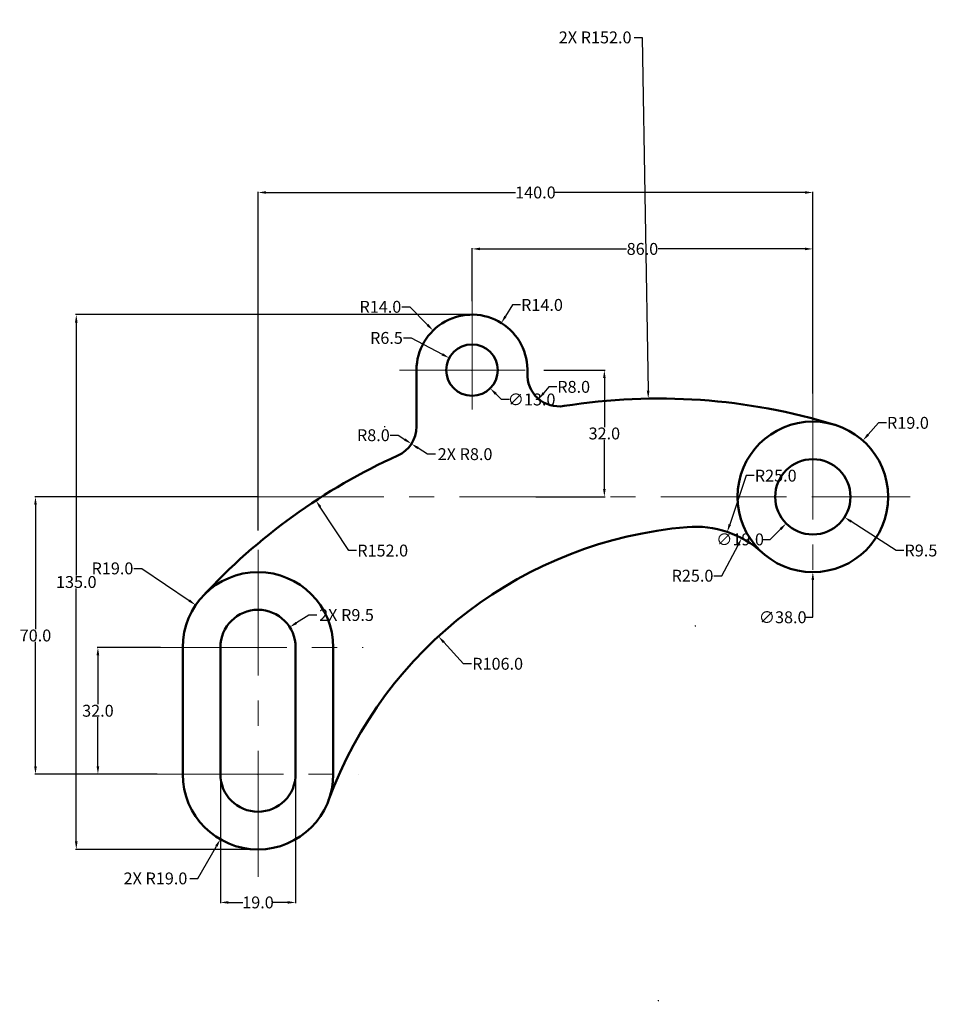
# Model space of a CAD drawing. Units: inches. Extents: x 66 to 297, y 17 to 265.
import ezdxf

# ---------------------------------------------------------------- set-up
doc = ezdxf.new("R2010")
doc.units = ezdxf.units.IN
doc.header["$MEASUREMENT"] = 0
doc.linetypes.add('CENTER', pattern=[50.8, 31.75, -6.35, 6.35, -6.35])
for name, color, linetype, lineweight in [('M-CNTR', 4, 'CENTER', 18), ('M-DIMS', 2, 'Continuous', 25), ('M-OUTL', 7, 'Continuous', 50)]:
    doc.layers.add(name, color=color, linetype=linetype, lineweight=lineweight)
doc.styles.get("Standard").update_dxf_attribs({"font": 'arial.ttf'})
doc.dimstyles.get("Standard").update_dxf_attribs({"dimtxt": 3, "dimasz": 2, "dimexe": 0.18, "dimexo": 0.0625, "dimgap": 0.09, "dimtad": 0, "dimtih": 1, "dimtoh": 1, "dimdec": 1, "dimzin": 0, "dimdsep": 46, "dimtxsty": 'Standard', "dimcen": 0.09, "dimclrd": 1, "dimclre": 1, "dimadec": 0, "dimazin": 0, "dimtfac": 1, "dimtdec": 1, "dimtofl": 0, "dimtmove": 0, "dimatfit": 3, "dimfxl": 1, "dimtolj": 1, "dimtzin": 0, "dimarcsym": 0})

# ---------------------------------------------------------------- blocks, each defined once
blk = doc.blocks.new('*D1')
at = {"layer": 'Defpoints', "color": 0, "transparency": 16777216}
for p in [(171.35, 109.8), (243.11, 31.78)]:
    blk.add_point(p, dxfattribs=at)
at = {"layer": 'M-DIMS', "color": 0, "lineweight": -2, "transparency": 16777216}
for p, q in [((177.72, 102.88), (172.71, 108.33)), ((179.72, 102.88), (177.72, 102.88))]:
    blk.add_line(p, q, dxfattribs=at)
at = {"layer": 'M-DIMS', "color": 0, "transparency": 16777216}
blk.add_solid([(172.95, 108.55), (172.46, 108.1), (171.35, 109.8)], dxfattribs=at)
at = {"layer": 'M-DIMS', "color": 0, "transparency": 16777216, "insert": (186.3, 102.88), "char_height": 3, "attachment_point": 5}
blk.add_mtext('\\A1;R106.0', dxfattribs=at)
blk = doc.blocks.new('*D2')
at = {"layer": 'Defpoints', "color": 0, "transparency": 16777216}
for p in [(116.33, 75.02), (135.33, 75.02), (135.33, 42.63)]:
    blk.add_point(p, dxfattribs=at)
at = {"layer": 'M-DIMS', "color": 0, "lineweight": -2, "transparency": 16777216}
for p, q in [((116.33, 74.96), (116.33, 42.45)), ((135.33, 74.96), (135.33, 42.45)), ((118.33, 42.63), (121.99, 42.63)), ((133.33, 42.63), (129.67, 42.63))]:
    blk.add_line(p, q, dxfattribs=at)
at = {"layer": 'M-DIMS', "color": 0, "transparency": 16777216}
for points in [[(118.33, 42.96), (118.33, 42.3), (116.33, 42.63)], [(133.33, 42.96), (133.33, 42.3), (135.33, 42.63)]]:
    blk.add_solid(points, dxfattribs=at)
at = {"layer": 'M-DIMS', "color": 0, "transparency": 16777216, "insert": (125.83, 42.63), "char_height": 3, "attachment_point": 5}
blk.add_mtext('\\A1;19.0', dxfattribs=at)
blk = doc.blocks.new('*D3')
at = {"layer": 'Defpoints', "color": 0, "transparency": 16777216}
for p in [(85.44, 107.02), (101.33, 107.02), (100.48, 75.02)]:
    blk.add_point(p, dxfattribs=at)
at = {"layer": 'M-DIMS', "color": 0, "lineweight": -2, "transparency": 16777216}
for p, q in [((101.27, 107.02), (85.26, 107.02)), ((85.44, 105.02), (85.44, 92.65)), ((85.44, 77.02), (85.44, 89.4)), ((100.42, 75.02), (85.26, 75.02))]:
    blk.add_line(p, q, dxfattribs=at)
at = {"layer": 'M-DIMS', "color": 0, "transparency": 16777216}
for points in [[(85.1, 105.02), (85.77, 105.02), (85.44, 107.02)], [(85.1, 77.02), (85.77, 77.02), (85.44, 75.02)]]:
    blk.add_solid(points, dxfattribs=at)
at = {"layer": 'M-DIMS', "color": 0, "transparency": 16777216, "insert": (85.44, 91.02), "char_height": 3, "attachment_point": 5}
blk.add_mtext('\\A1;32.0', dxfattribs=at)
blk = doc.blocks.new('*D4')
at = {"layer": 'Defpoints', "color": 0, "transparency": 16777216}
for p in [(125.83, 145.02), (69.68, 75.02), (100.48, 75.02)]:
    blk.add_point(p, dxfattribs=at)
at = {"layer": 'M-DIMS', "color": 0, "lineweight": -2, "transparency": 16777216}
for p, q in [((125.76, 145.02), (69.5, 145.02)), ((69.68, 143.02), (69.68, 111.64)), ((69.68, 77.02), (69.68, 108.4)), ((100.42, 75.02), (69.5, 75.02))]:
    blk.add_line(p, q, dxfattribs=at)
at = {"layer": 'M-DIMS', "color": 0, "transparency": 16777216}
for points in [[(69.35, 143.02), (70.01, 143.02), (69.68, 145.02)], [(69.35, 77.02), (70.01, 77.02), (69.68, 75.02)]]:
    blk.add_solid(points, dxfattribs=at)
at = {"layer": 'M-DIMS', "color": 0, "transparency": 16777216, "insert": (69.68, 110.02), "char_height": 3, "attachment_point": 5}
blk.add_mtext('\\A1;70.0', dxfattribs=at)
blk = doc.blocks.new('*D5')
at = {"layer": 'Defpoints', "color": 0, "transparency": 16777216}
for p in [(110.12, 117.71), (125.83, 107.02)]:
    blk.add_point(p, dxfattribs=at)
at = {"layer": 'M-DIMS', "color": 0, "lineweight": -2, "transparency": 16777216}
for p, q in [((94.52, 126.96), (96.52, 126.96)), ((96.52, 126.96), (108.46, 118.84)), ((125.74, 107.02), (125.92, 107.02)), ((125.83, 106.93), (125.83, 107.11))]:
    blk.add_line(p, q, dxfattribs=at)
at = {"layer": 'M-DIMS', "color": 0, "transparency": 16777216}
blk.add_solid([(108.65, 119.11), (108.28, 118.56), (110.12, 117.71)], dxfattribs=at)
at = {"layer": 'M-DIMS', "color": 0, "transparency": 16777216, "insert": (89.11, 126.96), "char_height": 3, "attachment_point": 5}
blk.add_mtext('\\A1;R19.0', dxfattribs=at)
blk = doc.blocks.new('*D6')
at = {"layer": 'Defpoints', "color": 0, "transparency": 16777216}
for p in [(140.44, 144.11), (223.65, 16.91)]:
    blk.add_point(p, dxfattribs=at)
at = {"layer": 'M-DIMS', "color": 0, "lineweight": -2, "transparency": 16777216}
for p, q in [((148.71, 131.46), (141.53, 142.44)), ((150.71, 131.46), (148.71, 131.46))]:
    blk.add_line(p, q, dxfattribs=at)
at = {"layer": 'M-DIMS', "color": 0, "transparency": 16777216}
blk.add_solid([(141.81, 142.62), (141.25, 142.26), (140.44, 144.11)], dxfattribs=at)
at = {"layer": 'M-DIMS', "color": 0, "transparency": 16777216, "insert": (157.29, 131.46), "char_height": 3, "attachment_point": 5}
blk.add_mtext('\\A1;R152.0', dxfattribs=at)
blk = doc.blocks.new('*D7')
at = {"layer": 'Defpoints', "color": 0, "transparency": 16777216}
for p in [(157.83, 162.74), (164.55, 158.41)]:
    blk.add_point(p, dxfattribs=at)
at = {"layer": 'M-DIMS', "color": 0, "lineweight": -2, "transparency": 16777216}
for p, q in [((159.19, 160.58), (161.19, 160.58)), ((161.19, 160.58), (162.87, 159.5))]:
    blk.add_line(p, q, dxfattribs=at)
at = {"layer": 'M-DIMS', "color": 0, "transparency": 16777216}
blk.add_solid([(163.05, 159.78), (162.69, 159.22), (164.55, 158.41)], dxfattribs=at)
at = {"layer": 'M-DIMS', "color": 0, "transparency": 16777216, "insert": (154.94, 160.58), "char_height": 3, "attachment_point": 5}
blk.add_mtext('\\A1;R8.0', dxfattribs=at)
blk = doc.blocks.new('*D8')
at = {"layer": 'Defpoints', "color": 0, "transparency": 16777216}
for p in [(174.08, 180.07), (179.83, 177.02)]:
    blk.add_point(p, dxfattribs=at)
at = {"layer": 'M-DIMS', "color": 0, "lineweight": -2, "transparency": 16777216}
for p, q in [((162.51, 185.14), (164.51, 185.14)), ((164.51, 185.14), (172.32, 181)), ((179.74, 177.02), (179.92, 177.02)), ((179.83, 176.93), (179.83, 177.11))]:
    blk.add_line(p, q, dxfattribs=at)
at = {"layer": 'M-DIMS', "color": 0, "transparency": 16777216}
blk.add_solid([(172.47, 181.3), (172.16, 180.71), (174.08, 180.07)], dxfattribs=at)
at = {"layer": 'M-DIMS', "color": 0, "transparency": 16777216, "insert": (158.24, 185.14), "char_height": 3, "attachment_point": 5}
blk.add_mtext('\\A1;R6.5', dxfattribs=at)
blk = doc.blocks.new('*D9')
at = {"layer": 'Defpoints', "color": 0, "transparency": 16777216}
for p in [(187.22, 188.91), (179.83, 177.02)]:
    blk.add_point(p, dxfattribs=at)
at = {"layer": 'M-DIMS', "color": 0, "lineweight": -2, "transparency": 16777216}
for p, q in [((190.06, 193.47), (188.28, 190.61)), ((192.06, 193.47), (190.06, 193.47)), ((179.74, 177.02), (179.92, 177.02)), ((179.83, 176.93), (179.83, 177.11))]:
    blk.add_line(p, q, dxfattribs=at)
at = {"layer": 'M-DIMS', "color": 0, "transparency": 16777216}
blk.add_solid([(188, 190.78), (188.56, 190.43), (187.22, 188.91)], dxfattribs=at)
at = {"layer": 'M-DIMS', "color": 0, "transparency": 16777216, "insert": (197.48, 193.47), "char_height": 3, "attachment_point": 5}
blk.add_mtext('\\A1;R14.0', dxfattribs=at)
blk = doc.blocks.new('*D10')
at = {"layer": 'Defpoints', "color": 0, "transparency": 16777216}
for p in [(201.79, 175.86), (196.66, 169.72)]:
    blk.add_point(p, dxfattribs=at)
at = {"layer": 'M-DIMS', "color": 0, "lineweight": -2, "transparency": 16777216}
for p, q in [((199.23, 172.79), (197.95, 171.25)), ((201.23, 172.79), (199.23, 172.79))]:
    blk.add_line(p, q, dxfattribs=at)
at = {"layer": 'M-DIMS', "color": 0, "transparency": 16777216}
blk.add_solid([(197.69, 171.47), (198.2, 171.04), (196.66, 169.72)], dxfattribs=at)
at = {"layer": 'M-DIMS', "color": 0, "transparency": 16777216, "insert": (205.48, 172.79), "char_height": 3, "attachment_point": 5}
blk.add_mtext('\\A1;R8.0', dxfattribs=at)
blk = doc.blocks.new('*D11')
at = {"layer": 'Defpoints', "color": 0, "transparency": 16777216}
for p in [(197.89, 177.02), (195.83, 145.02), (213.22, 145.02)]:
    blk.add_point(p, dxfattribs=at)
at = {"layer": 'M-DIMS', "color": 0, "lineweight": -2, "transparency": 16777216}
for p, q in [((197.96, 177.02), (213.4, 177.02)), ((213.22, 175.02), (213.22, 162.65)), ((213.22, 147.02), (213.22, 159.4)), ((195.89, 145.02), (213.4, 145.02))]:
    blk.add_line(p, q, dxfattribs=at)
at = {"layer": 'M-DIMS', "color": 0, "transparency": 16777216}
for points in [[(212.89, 175.02), (213.55, 175.02), (213.22, 177.02)], [(212.89, 147.02), (213.55, 147.02), (213.22, 145.02)]]:
    blk.add_solid(points, dxfattribs=at)
at = {"layer": 'M-DIMS', "color": 0, "transparency": 16777216, "insert": (213.22, 161.02), "char_height": 3, "attachment_point": 5}
blk.add_mtext('\\A1;32.0', dxfattribs=at)
blk = doc.blocks.new('*D12')
at = {"layer": 'Defpoints', "color": 0, "transparency": 16777216}
for p in [(247.88, 134.59), (236.21, 112.48)]:
    blk.add_point(p, dxfattribs=at)
at = {"layer": 'M-DIMS', "color": 0, "lineweight": -2, "transparency": 16777216}
for p, q in [((242.87, 125.11), (246.95, 132.82)), ((240.87, 125.11), (242.87, 125.11))]:
    blk.add_line(p, q, dxfattribs=at)
at = {"layer": 'M-DIMS', "color": 0, "transparency": 16777216}
blk.add_solid([(246.65, 132.98), (247.24, 132.67), (247.88, 134.59)], dxfattribs=at)
at = {"layer": 'M-DIMS', "color": 0, "transparency": 16777216, "insert": (235.46, 125.11), "char_height": 3, "attachment_point": 5}
blk.add_mtext('\\A1;R25.0', dxfattribs=at)
blk = doc.blocks.new('*D13')
at = {"layer": 'Defpoints', "color": 0, "transparency": 16777216}
for p in [(265.83, 145.02), (273.81, 139.87)]:
    blk.add_point(p, dxfattribs=at)
at = {"layer": 'M-DIMS', "color": 0, "lineweight": -2, "transparency": 16777216}
for p, q in [((265.74, 145.02), (265.92, 145.02)), ((265.83, 144.93), (265.83, 145.11)), ((286.82, 131.48), (275.49, 138.79)), ((288.82, 131.48), (286.82, 131.48))]:
    blk.add_line(p, q, dxfattribs=at)
at = {"layer": 'M-DIMS', "color": 0, "transparency": 16777216}
blk.add_solid([(275.67, 139.07), (275.31, 138.51), (273.81, 139.87)], dxfattribs=at)
at = {"layer": 'M-DIMS', "color": 0, "transparency": 16777216, "insert": (293.09, 131.48), "char_height": 3, "attachment_point": 5}
blk.add_mtext('\\A1;R9.5', dxfattribs=at)
blk = doc.blocks.new('*D14')
at = {"layer": 'Defpoints', "color": 0, "transparency": 16777216}
for p in [(278.44, 159.23), (265.83, 145.02)]:
    blk.add_point(p, dxfattribs=at)
at = {"layer": 'M-DIMS', "color": 0, "lineweight": -2, "transparency": 16777216}
for p, q in [((282.4, 163.7), (279.77, 160.73)), ((284.4, 163.7), (282.4, 163.7)), ((265.74, 145.02), (265.92, 145.02)), ((265.83, 144.93), (265.83, 145.11))]:
    blk.add_line(p, q, dxfattribs=at)
at = {"layer": 'M-DIMS', "color": 0, "transparency": 16777216}
blk.add_solid([(279.52, 160.95), (280.02, 160.51), (278.44, 159.23)], dxfattribs=at)
at = {"layer": 'M-DIMS', "color": 0, "transparency": 16777216, "insert": (289.82, 163.7), "char_height": 3, "attachment_point": 5}
blk.add_mtext('\\A1;R19.0', dxfattribs=at)
blk = doc.blocks.new('*D15')
at = {"layer": 'Defpoints', "color": 0, "transparency": 16777216}
for p in [(265.83, 207.61), (179.83, 194.35), (265.83, 171.06)]:
    blk.add_point(p, dxfattribs=at)
at = {"layer": 'M-DIMS', "color": 0, "lineweight": -2, "transparency": 16777216}
for p, q in [((179.83, 194.41), (179.83, 207.79)), ((181.83, 207.61), (218.84, 207.61)), ((263.83, 207.61), (226.81, 207.61)), ((265.83, 171.13), (265.83, 207.79))]:
    blk.add_line(p, q, dxfattribs=at)
at = {"layer": 'M-DIMS', "color": 0, "transparency": 16777216}
for points in [[(181.83, 207.94), (181.83, 207.28), (179.83, 207.61)], [(263.83, 207.94), (263.83, 207.28), (265.83, 207.61)]]:
    blk.add_solid(points, dxfattribs=at)
at = {"layer": 'M-DIMS', "color": 0, "transparency": 16777216, "insert": (222.83, 207.61), "char_height": 3, "attachment_point": 5}
blk.add_mtext('\\A1;86.0', dxfattribs=at)
blk = doc.blocks.new('*D16')
at = {"layer": 'Defpoints', "color": 0, "transparency": 16777216}
for p in [(125.83, 221.86), (265.83, 171.06), (125.83, 136.5)]:
    blk.add_point(p, dxfattribs=at)
at = {"layer": 'M-DIMS', "color": 0, "lineweight": -2, "transparency": 16777216}
for p, q in [((125.83, 136.56), (125.83, 222.04)), ((127.83, 221.86), (190.82, 221.86)), ((263.83, 221.86), (200.83, 221.86)), ((265.83, 171.13), (265.83, 222.04))]:
    blk.add_line(p, q, dxfattribs=at)
at = {"layer": 'M-DIMS', "color": 0, "transparency": 16777216}
for points in [[(127.83, 222.19), (127.83, 221.53), (125.83, 221.86)], [(263.83, 222.19), (263.83, 221.53), (265.83, 221.86)]]:
    blk.add_solid(points, dxfattribs=at)
at = {"layer": 'M-DIMS', "color": 0, "transparency": 16777216, "insert": (195.83, 221.86), "char_height": 3, "attachment_point": 5}
blk.add_mtext('\\A1;140.0', dxfattribs=at)
blk = doc.blocks.new('*D17')
at = {"layer": 'Defpoints', "color": 0, "transparency": 16777216}
for p in [(79.98, 191.02), (180.2, 191.02), (125.83, 56.02)]:
    blk.add_point(p, dxfattribs=at)
at = {"layer": 'M-DIMS', "color": 1, "lineweight": -2, "transparency": 16777216}
for p, q in [((180.13, 191.02), (79.8, 191.02)), ((79.98, 189.02), (79.98, 125.14)), ((79.98, 58.02), (79.98, 121.9)), ((125.76, 56.02), (79.8, 56.02))]:
    blk.add_line(p, q, dxfattribs=at)
at = {"layer": 'M-DIMS', "color": 1, "transparency": 16777216}
for points in [[(79.65, 189.02), (80.31, 189.02), (79.98, 191.02)], [(79.65, 58.02), (80.31, 58.02), (79.98, 56.02)]]:
    blk.add_solid(points, dxfattribs=at)
at = {"layer": 'M-DIMS', "color": 0, "transparency": 16777216, "insert": (79.98, 123.52), "char_height": 3, "attachment_point": 5}
blk.add_mtext('\\A1;135.0', dxfattribs=at)
blk = doc.blocks.new('*D18')
at = {"layer": 'Defpoints', "color": 0, "transparency": 16777216}
for p in [(224.3, 169.82), (226.91, 17.84)]:
    blk.add_point(p, dxfattribs=at)
at = {"layer": 'M-DIMS', "color": 1, "lineweight": -2, "transparency": 16777216}
for p, q in [((220.73, 261.01), (222.73, 261.01)), ((222.73, 261.01), (224.27, 171.82)), ((226.82, 17.84), (227, 17.84)), ((226.91, 17.75), (226.91, 17.93))]:
    blk.add_line(p, q, dxfattribs=at)
at = {"layer": 'M-DIMS', "color": 1, "transparency": 16777216}
blk.add_solid([(224.6, 171.82), (223.93, 171.81), (224.3, 169.82)], dxfattribs=at)
at = {"layer": 'M-DIMS', "color": 0, "transparency": 16777216, "insert": (210.9, 261.01), "char_height": 3, "attachment_point": 5}
blk.add_mtext('\\A1;2X R152.0', dxfattribs=at)
blk = doc.blocks.new('*D19')
at = {"layer": 'Defpoints', "color": 0, "transparency": 16777216}
for p in [(244.23, 136.16), (236.21, 112.48)]:
    blk.add_point(p, dxfattribs=at)
at = {"layer": 'M-DIMS', "color": 1, "lineweight": -2, "transparency": 16777216}
for p, q in [((249.04, 150.37), (244.87, 138.06)), ((251.04, 150.37), (249.04, 150.37)), ((236.12, 112.48), (236.3, 112.48)), ((236.21, 112.39), (236.21, 112.57))]:
    blk.add_line(p, q, dxfattribs=at)
at = {"layer": 'M-DIMS', "color": 1, "transparency": 16777216}
blk.add_solid([(244.55, 138.16), (245.18, 137.95), (244.23, 136.16)], dxfattribs=at)
at = {"layer": 'M-DIMS', "color": 0, "transparency": 16777216, "insert": (256.46, 150.37), "char_height": 3, "attachment_point": 5}
blk.add_mtext('\\A1;R25.0', dxfattribs=at)
blk = doc.blocks.new('*D20')
at = {"layer": 'Defpoints', "color": 0, "transparency": 16777216}
for p in [(125.83, 75.02), (116.33, 58.57)]:
    blk.add_point(p, dxfattribs=at)
at = {"layer": 'M-DIMS', "color": 1, "lineweight": -2, "transparency": 16777216}
for p, q in [((125.74, 75.02), (125.92, 75.02)), ((125.83, 74.93), (125.83, 75.11)), ((110.63, 48.69), (115.33, 56.84)), ((108.63, 48.69), (110.63, 48.69))]:
    blk.add_line(p, q, dxfattribs=at)
at = {"layer": 'M-DIMS', "color": 1, "transparency": 16777216}
blk.add_solid([(115.04, 57), (115.61, 56.67), (116.33, 58.57)], dxfattribs=at)
at = {"layer": 'M-DIMS', "color": 0, "transparency": 16777216, "insert": (99.96, 48.69), "char_height": 3, "attachment_point": 5}
blk.add_mtext('\\A1;2X R19.0', dxfattribs=at)
blk = doc.blocks.new('*D21')
at = {"layer": 'Defpoints', "color": 0, "transparency": 16777216}
for p in [(265.82, 164.02), (265.82, 126.02)]:
    blk.add_point(p, dxfattribs=at)
at = {"layer": 'M-DIMS', "color": 1, "lineweight": -2, "transparency": 16777216}
for p, q in [((265.74, 145.02), (265.92, 145.02)), ((265.82, 144.93), (265.82, 145.11)), ((265.82, 114.62), (265.82, 124.02)), ((263.82, 114.62), (265.82, 114.62))]:
    blk.add_line(p, q, dxfattribs=at)
at = {"layer": 'M-DIMS', "color": 1, "transparency": 16777216}
blk.add_solid([(265.49, 124.02), (266.16, 124.02), (265.82, 126.02)], dxfattribs=at)
at = {"layer": 'M-DIMS', "color": 0, "transparency": 16777216, "insert": (258.21, 114.62), "char_height": 3, "attachment_point": 5}
blk.add_mtext('\\A1;∅38.0', dxfattribs=at)
blk = doc.blocks.new('*D22')
at = {"layer": 'Defpoints', "color": 0, "transparency": 16777216}
for p in [(170.01, 187.01), (179.83, 177.02)]:
    blk.add_point(p, dxfattribs=at)
at = {"layer": 'M-DIMS', "color": 1, "lineweight": -2, "transparency": 16777216}
for p, q in [((162.12, 193), (164.12, 193)), ((164.12, 193), (168.61, 188.43)), ((179.74, 177.02), (179.92, 177.02)), ((179.83, 176.93), (179.83, 177.11))]:
    blk.add_line(p, q, dxfattribs=at)
at = {"layer": 'M-DIMS', "color": 1, "transparency": 16777216}
blk.add_solid([(168.85, 188.67), (168.37, 188.2), (170.01, 187.01)], dxfattribs=at)
at = {"layer": 'M-DIMS', "color": 0, "transparency": 16777216, "insert": (156.71, 193), "char_height": 3, "attachment_point": 5}
blk.add_mtext('\\A1;R14.0', dxfattribs=at)
blk = doc.blocks.new('*D23')
at = {"layer": 'Defpoints', "color": 0, "transparency": 16777216}
for p in [(133.84, 112.12), (125.83, 107.02)]:
    blk.add_point(p, dxfattribs=at)
at = {"layer": 'M-DIMS', "color": 1, "lineweight": -2, "transparency": 16777216}
for p, q in [((138.65, 115.19), (135.53, 113.2)), ((140.65, 115.19), (138.65, 115.19)), ((125.74, 107.02), (125.92, 107.02)), ((125.83, 106.93), (125.83, 107.11))]:
    blk.add_line(p, q, dxfattribs=at)
at = {"layer": 'M-DIMS', "color": 1, "transparency": 16777216}
blk.add_solid([(135.35, 113.48), (135.7, 112.92), (133.84, 112.12)], dxfattribs=at)
at = {"layer": 'M-DIMS', "color": 0, "transparency": 16777216, "insert": (148.16, 115.19), "char_height": 3, "attachment_point": 5}
blk.add_mtext('\\A1;2X R9.5', dxfattribs=at)
blk = doc.blocks.new('*D24')
at = {"layer": 'Defpoints', "color": 0, "transparency": 16777216}
for p in [(272.54, 151.74), (259.11, 138.31)]:
    blk.add_point(p, dxfattribs=at)
at = {"layer": 'M-DIMS', "color": 1, "lineweight": -2, "transparency": 16777216}
for p, q in [((265.74, 145.02), (265.92, 145.02)), ((265.83, 144.93), (265.83, 145.11)), ((255.07, 134.28), (257.69, 136.89)), ((253.07, 134.28), (255.07, 134.28))]:
    blk.add_line(p, q, dxfattribs=at)
at = {"layer": 'M-DIMS', "color": 1, "transparency": 16777216}
blk.add_solid([(257.46, 137.13), (257.93, 136.66), (259.11, 138.31)], dxfattribs=at)
at = {"layer": 'M-DIMS', "color": 0, "transparency": 16777216, "insert": (247.46, 134.28), "char_height": 3, "attachment_point": 5}
blk.add_mtext('\\A1;∅19.0', dxfattribs=at)
blk = doc.blocks.new('*D25')
at = {"layer": 'Defpoints', "color": 0, "transparency": 16777216}
for p in [(157.83, 162.74), (164.55, 158.4)]:
    blk.add_point(p, dxfattribs=at)
at = {"layer": 'M-DIMS', "color": 1, "lineweight": -2, "transparency": 16777216}
for p, q in [((157.74, 162.74), (157.92, 162.74)), ((157.83, 162.65), (157.83, 162.83)), ((168.58, 155.8), (166.23, 157.32)), ((170.58, 155.8), (168.58, 155.8))]:
    blk.add_line(p, q, dxfattribs=at)
at = {"layer": 'M-DIMS', "color": 1, "transparency": 16777216}
blk.add_solid([(166.41, 157.6), (166.04, 157.04), (164.55, 158.4)], dxfattribs=at)
at = {"layer": 'M-DIMS', "color": 0, "transparency": 16777216, "insert": (178.08, 155.8), "char_height": 3, "attachment_point": 5}
blk.add_mtext('\\A1;2X R8.0', dxfattribs=at)
blk = doc.blocks.new('*D26')
at = {"layer": 'Defpoints', "color": 0, "transparency": 16777216}
for p in [(175.23, 181.62), (184.42, 172.42)]:
    blk.add_point(p, dxfattribs=at)
at = {"layer": 'M-DIMS', "color": 1, "lineweight": -2, "transparency": 16777216}
for p, q in [((179.74, 177.02), (179.92, 177.02)), ((179.83, 176.93), (179.83, 177.11)), ((187.25, 169.6), (185.83, 171.01)), ((189.25, 169.6), (187.25, 169.6))]:
    blk.add_line(p, q, dxfattribs=at)
at = {"layer": 'M-DIMS', "color": 1, "transparency": 16777216}
blk.add_solid([(186.07, 171.25), (185.6, 170.77), (184.42, 172.42)], dxfattribs=at)
at = {"layer": 'M-DIMS', "color": 0, "transparency": 16777216, "insert": (194.86, 169.6), "char_height": 3, "attachment_point": 5}
blk.add_mtext('\\A1;∅13.0', dxfattribs=at)

msp = doc.modelspace()

# ---------------------------------------------------------------- linework, layer by layer
at = {"layer": 'M-CNTR'}
for p, q in [((179.83, 194.35), (179.83, 167.05)), ((161.5, 177.02), (197.89, 177.02)), ((265.82, 171.06), (265.82, 118.07)), ((125.83, 145.02), (265.82, 145.02)), ((265.82, 145.02), (290.39, 145.02)), ((125.83, 49.13), (125.83, 136.5)), ((101.33, 107.02), (152.38, 107.02)), ((100.48, 75.02), (151.31, 75.02))]:
    msp.add_line(p, q, dxfattribs=at)
at = {"layer": 'M-OUTL'}
for p, q in [((165.83, 177.02), (165.83, 162.74)), ((106.83, 75.02), (106.83, 107.02)), ((116.33, 75.02), (116.33, 107.02)), ((135.33, 75.02), (135.33, 107.02)), ((144.83, 75.02), (144.83, 107.02))]:
    msp.add_line(p, q, dxfattribs=at)
for centre, radius in [((179.83, 177.02), 6.5), ((265.82, 145.02), 19), ((265.82, 145.02), 9.5)]:
    msp.add_circle(centre, radius, dxfattribs=at)
for centre, radius, start, end in [((179.83, 177.02), 14, 356.9639, 180), ((201.79, 175.86), 8, 176.9639, 279.033), ((226.91, 17.84), 152, 72.9888, 99.033), ((157.83, 162.74), 8, 294.2915, 0), ((223.65, 16.91), 152, 114.2915, 137.349), ((243.11, 31.78), 106, 94.887, 159.7602), ((236.21, 112.48), 25, 47.6891, 94.887), ((125.83, 107.02), 19, 0, 180), ((125.83, 107.02), 9.5, 0, 180), ((125.83, 75.02), 19, 180, 0), ((125.83, 75.02), 9.5, 180, 0)]:
    msp.add_arc(centre, radius, start, end, dxfattribs=at)

# ---------------------------------------------------------------- dimensions: what is measured, and where the dimension line sits
at = {"layer": 'M-DIMS'}
for center, mpoint, picture, middle in [((226.91, 17.84), (224.3, 169.82), '*D18', (210.9, 261.01)), ((157.83, 162.74), (164.55, 158.4), '*D25', (178.08, 155.8)), ((125.83, 107.02), (133.84, 112.12), '*D23', (148.16, 115.19)), ((125.83, 75.02), (116.33, 58.57), '*D20', (99.96, 48.69))]:
    dim = msp.add_radius_dim(center=center, mpoint=mpoint, text='2X <>', dimstyle='Standard', override={"dimdec": 1, "dimlfac": 1, "dimrnd": 0, "dimzin": 0, "dimdsep": 46, "dimlunit": 2}, dxfattribs=at)
    dim.commit()
    dim.dimension.update_dxf_attribs({"geometry": picture, "text_midpoint": middle, "dimtype": 164})
for base, p1, p2, picture, middle in [((125.83, 221.86), (265.82, 171.06), (125.83, 136.5), '*D16', (195.83, 221.86)), ((265.82, 207.61), (179.83, 194.35), (265.82, 171.06), '*D15', (222.83, 207.61)), ((135.33, 42.63), (116.33, 75.02), (135.33, 75.02), '*D2', (125.83, 42.63))]:
    dim = msp.add_linear_dim(base=base, p1=p1, p2=p2, dimstyle='Standard', override={"dimclrd": 0, "dimclre": 0, "dimclrt": 0}, dxfattribs=at)
    dim.commit()
    dim.dimension.update_dxf_attribs({"geometry": picture, "text_midpoint": middle})
for center, mpoint, override, picture, middle in [((179.83, 177.02), (170.01, 187.01), {"dimdec": 1, "dimlfac": 1, "dimrnd": 0, "dimzin": 0, "dimdsep": 46, "dimlunit": 2}, '*D22', (156.71, 193)), ((179.83, 177.02), (187.22, 188.91), {"dimclrd": 0, "dimclre": 0, "dimclrt": 0}, '*D9', (197.48, 193.47)), ((179.83, 177.02), (174.08, 180.07), {"dimclrd": 0, "dimclre": 0, "dimclrt": 0}, '*D8', (158.24, 185.14)), ((201.79, 175.86), (196.66, 169.72), {"dimclrd": 0, "dimclre": 0, "dimclrt": 0}, '*D10', (205.48, 172.79)), ((265.82, 145.02), (278.44, 159.23), {"dimclrd": 0, "dimclre": 0, "dimclrt": 0}, '*D14', (289.82, 163.7)), ((157.83, 162.74), (164.55, 158.41), {"dimclrd": 0, "dimclre": 0, "dimclrt": 0}, '*D7', (154.94, 160.58)), ((236.21, 112.48), (244.23, 136.16), {"dimdec": 1, "dimlfac": 1, "dimrnd": 0, "dimzin": 0, "dimdsep": 46, "dimlunit": 2}, '*D19', (256.46, 150.37)), ((265.82, 145.02), (273.81, 139.87), {"dimclrd": 0, "dimclre": 0, "dimclrt": 0}, '*D13', (293.09, 131.48)), ((223.65, 16.91), (140.44, 144.11), {"dimclrd": 0, "dimclre": 0, "dimclrt": 0}, '*D6', (157.29, 131.46)), ((236.21, 112.48), (247.88, 134.59), {"dimclrd": 0, "dimclre": 0, "dimclrt": 0}, '*D12', (235.46, 125.11)), ((125.83, 107.02), (110.12, 117.71), {"dimclrd": 0, "dimclre": 0, "dimclrt": 0}, '*D5', (89.11, 126.96)), ((243.11, 31.78), (171.35, 109.8), {"dimclrd": 0, "dimclre": 0, "dimclrt": 0}, '*D1', (186.3, 102.88))]:
    dim = msp.add_radius_dim(center=center, mpoint=mpoint, dimstyle='Standard', override=override, dxfattribs=at)
    dim.commit()
    dim.dimension.update_dxf_attribs({"geometry": picture, "text_midpoint": middle, "dimtype": 164})
for base, p1, p2, override, picture, middle in [((79.98, 191.02), (125.83, 56.02), (180.2, 191.02), {"dimdec": 1, "dimlfac": 1, "dimrnd": 0, "dimzin": 0, "dimdsep": 46, "dimlunit": 2}, '*D17', (79.98, 123.52)), ((213.22, 145.02), (197.89, 177.02), (195.83, 145.02), {"dimclrd": 0, "dimclre": 0, "dimclrt": 0}, '*D11', (213.22, 161.02)), ((69.68, 75.02), (125.83, 145.02), (100.48, 75.02), {"dimclrd": 0, "dimclre": 0, "dimclrt": 0}, '*D4', (69.68, 110.02)), ((85.44, 107.02), (100.48, 75.02), (101.33, 107.02), {"dimclrd": 0, "dimclre": 0, "dimclrt": 0}, '*D3', (85.44, 91.02))]:
    dim = msp.add_linear_dim(base=base, p1=p1, p2=p2, angle=90, dimstyle='Standard', override=override, dxfattribs=at)
    dim.commit()
    dim.dimension.update_dxf_attribs({"geometry": picture, "text_midpoint": middle})
for p1, p2, picture, middle in [((175.23, 181.62), (184.42, 172.42), '*D26', (194.86, 169.6)), ((265.82, 164.02), (265.82, 126.02), '*D21', (258.21, 114.62)), ((272.54, 151.74), (259.11, 138.31), '*D24', (247.46, 134.28))]:
    dim = msp.add_diameter_dim_2p(p1=p1, p2=p2, dimstyle='Standard', override={"dimdec": 1, "dimlfac": 1, "dimrnd": 0, "dimzin": 0, "dimdsep": 46, "dimlunit": 2}, dxfattribs=at)
    dim.commit()
    dim.dimension.update_dxf_attribs({"geometry": picture, "text_midpoint": middle, "dimtype": 163})

doc.saveas('drawing.dxf')
